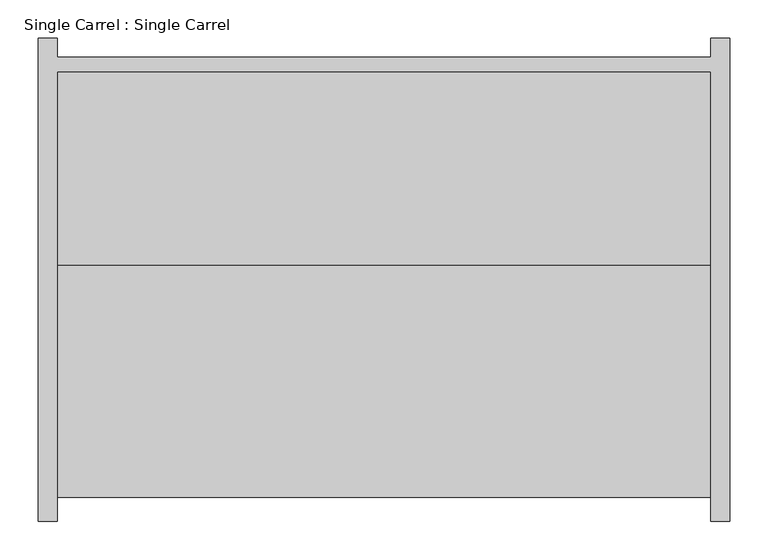
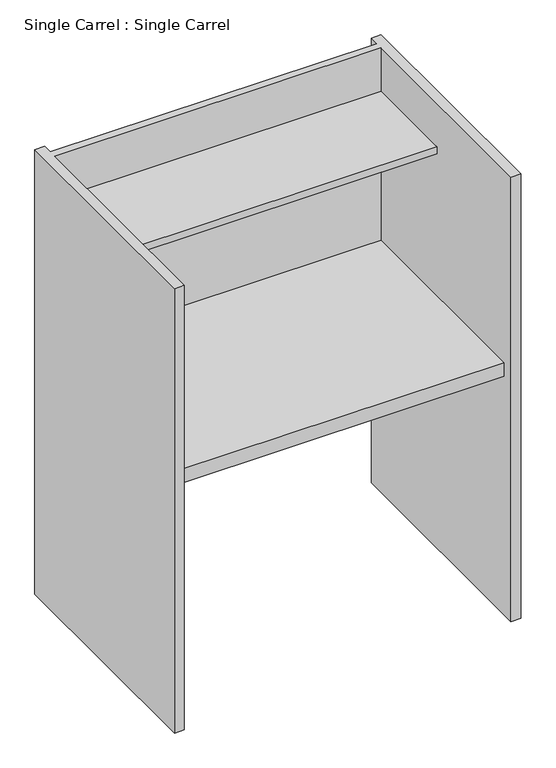
"""IFC4 building model written with IfcOpenShell, lengths in millimetres: proxy geometry, Single Carrel : Single Carrel."""

from ifc_helpers import new_model, si_unit, frame, origin, place, context, project, spatial, polyline, outline, extrude, faceted_brep, source, transform, mapped, element, save


def single_carrel_single_carrel_ed4d160c(model_context):
    return source(origin(), model_context, "Body", "SolidModel", [
        extrude(outline(polyline([(428.625, -19.05), (428.625, -273.05), (-428.625, -273.05), (-428.625, -19.05), (428.625, -19.05)])), frame((0.0, 0.0, 1092.2), z_axis=(0.0, 0.0, 1.0), x_axis=(1.0, 0.0, 0.0)), (0.0, 0.0, 1.0), 19.05),
        extrude(outline(polyline([(428.625, -19.05), (428.625, -577.85), (-428.625, -577.85), (-428.625, -19.05), (428.625, -19.05)])), frame((0.0, 0.0, 660.4), z_axis=(0.0, 0.0, 1.0), x_axis=(1.0, 0.0, 0.0)), (0.0, 0.0, 1.0), 38.1),
        faceted_brep([(428.625, 0.0, 1231.9), (-428.625, 0.0, 1231.9), (-428.625, 25.4, 1231.9), (-454.025, 25.4, 1231.9), (-454.025, -609.6, 1231.9), (-428.625, -609.6, 1231.9), (-428.625, -19.05, 1231.9), (428.625, -19.05, 1231.9), (428.625, -609.6, 1231.9), (454.025, -609.6, 1231.9), (454.025, 25.4, 1231.9), (428.625, 25.4, 1231.9), (428.625, -609.6, 0.0), (428.625, 25.4, 0.0), (454.025, 25.4, 0.0), (454.025, -609.6, 0.0), (-428.625, 25.4, 0.0), (-428.625, -609.6, 0.0), (-454.025, -609.6, 0.0), (-454.025, 25.4, 0.0), (428.625, 0.0, 457.2), (-428.625, 0.0, 457.2), (-428.625, -19.05, 457.2), (428.625, -19.05, 457.2)], [[[0, 1, 2, 3, 4, 5, 6, 7, 8, 9, 10, 11]], [[12, 13, 14, 15]], [[16, 17, 18, 19]], [[1, 0, 20, 21]], [[2, 1, 21, 22, 6, 5, 17, 16]], [[3, 2, 16, 19]], [[4, 3, 19, 18]], [[5, 4, 18, 17]], [[7, 6, 22, 23]], [[8, 7, 23, 20, 0, 11, 13, 12]], [[9, 8, 12, 15]], [[10, 9, 15, 14]], [[13, 11, 10, 14]], [[22, 21, 20, 23]]]),
    ])


if __name__ == "__main__":
    model = new_model("IFC4")
    model_context = context("Model", 3, world=origin())
    ifc_project = project(units=[si_unit("LENGTHUNIT", "METRE", prefix="MILLI")], contexts=[model_context])
    site = spatial("IfcSite", under=ifc_project)
    building = spatial("IfcBuilding", under=site)
    placement = place(None, origin())
    single_carrel_single_carrel_shape = single_carrel_single_carrel_ed4d160c(model_context)
    element("IfcBuildingElementProxy", 1, Name="Single Carrel : Single Carrel", ObjectType="Single Carrel : Single Carrel", at=placement, inside=building, context=model_context, shape_type="MappedRepresentation", body=[
        mapped(single_carrel_single_carrel_shape, transform((0.0, 0.0, 0.0), x_axis=(1.0, 0.0, 0.0), y_axis=(0.0, 1.0, 0.0), z_axis=(0.0, 0.0, 1.0))),
    ])
    save(model, "model.ifc")

# Revit data of these elements
# Type "Single Carrel : Single Carrel"
#   Assembly Code = "E1020200"
#   Width = 2' - 11 3/4"
#   Carrel Material = Laminate, Ivory, Matte
#   Desktop/Shelf Material = Cherry
#   Default Elevation = 0
# Element 1 (IfcBuildingElementProxy, "Single Carrel : Single Carrel")
#   Materials on its faces: "Laminate, Ivory, Matte", "Cherry"
# Materials
#   "Laminate, Ivory, Matte": class "Plastic", colour RGB 247 247 239, transparency 0, Description = "Plastic Laminate - Ivory, Matte", Cost = 0
#   "Cherry": class "Wood", colour RGB 226 177 128, transparency 0, Description = "Prunus Serotina", Cost = 0
